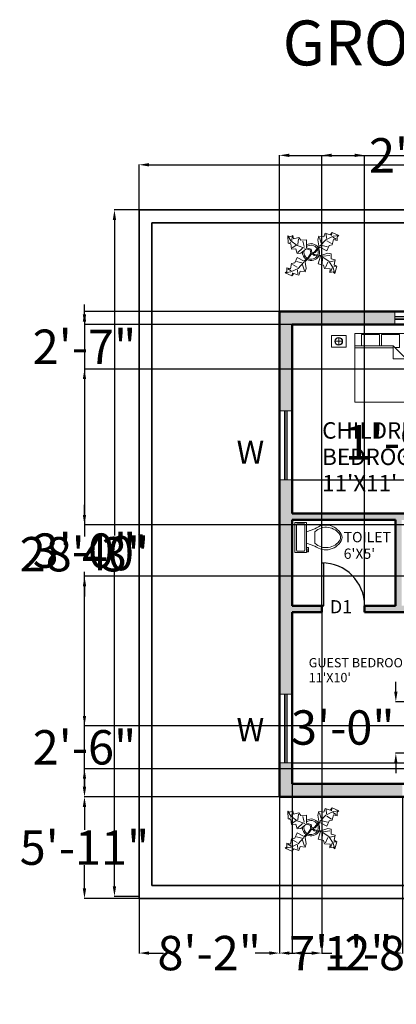
# Model space of a CAD drawing. Units: inches. Extents: x -166 to 1001, y 0 to 688.
# Tile 1 of 11: x -166 to 97, y 0 to 688. Entities that reach past the tile are written whole.
import ezdxf

# ---------------------------------------------------------------- set-up
doc = ezdxf.new("R2010")
doc.units = ezdxf.units.IN
doc.header["$MEASUREMENT"] = 0
for name, color, linetype, lineweight in [('A-ANNO-DIMS', 1, 'Continuous', 18), ('A-ANNO-TEXT', 2, 'Continuous', 25), ('A-AREA-IDEN', 2, 'Continuous', 25), ('A-DOOR', 6, 'Continuous', 25), ('A-FLOR-FIXT', 11, 'Continuous', 18), ('A-GLAZ', 130, 'Continuous', 18), ('A-WALL-PATT', 5, 'Continuous', 13), ('C-SITE-WALL', 250, 'Continuous', 35), ('FURNITURE', 11, 'Continuous', 18), ('TREES', 80, 'Continuous', 13), ('WALLS', 250, 'Continuous', 50)]:
    doc.layers.add(name, color=color, linetype=linetype, lineweight=lineweight)
doc.styles.get("Standard").update_dxf_attribs({"font": 'arial.ttf'})
doc.dimstyles.get("Standard").update_dxf_attribs({"dimtxt": 24, "dimasz": 7, "dimexe": 0.18, "dimexo": 0.0625, "dimgap": 0.09, "dimtad": 0, "dimtih": 1, "dimtoh": 1, "dimdec": 0, "dimzin": 0, "dimdsep": 46, "dimlunit": 3, "dimtxsty": 'Standard', "dimcen": 0.09, "dimadec": 0, "dimazin": 0, "dimtfac": 1, "dimtdec": 0, "dimtofl": 0, "dimtmove": 0, "dimatfit": 3, "dimfxl": 1, "dimtolj": 1, "dimtzin": 0, "dimarcsym": 0})

# ---------------------------------------------------------------- blocks, each defined once
blk = doc.blocks.new('*U6')
for p, q in [((0, 0), (0, -6)), ((40, 0), (40, -6))]:
    blk.add_line(p, q)
blk.add_lwpolyline([(0, 0), (0, 40), (1.75, 40), (1.75, 0)], close=True)
blk.add_arc((0, 0), 40, 0, 90)
blk = doc.blocks.new('Bed - Queen')
for p, q in [((0, -80.00003), (0, 0)), ((0, 0), (59.99999, 0)), ((59.99999, 0), (59.99999, -80.00003)), ((7.99999, -1.2), (28.79998, -1.2)), ((7.99999, -14.4), (7.99999, -1.2)), ((28.79998, -1.2), (28.79998, -14.4)), ((31.19999, -1.2), (51.99999, -1.2)), ((31.19999, -14.4), (31.19999, -1.2)), ((51.99999, -1.2), (51.99999, -16.4)), ((0, -14.4), (44.8, -14.4)), ((44.8, -16.8), (0, -16.8)), ((59.99999, -29.6), (44.8, -14.4)), ((44.8, -14.4), (44.8, -29.6)), ((51.99999, -16.4), (46.79936, -16.4)), ((44.8, -29.6), (59.99999, -29.6)), ((59.99999, -80.00003), (0, -80.00003))]:
    blk.add_line(p, q)
blk = doc.blocks.new('Toilet - top')
for p, q in [((9.5, -6), (9.5, -2)), ((-10, -8.5), (-8, -8.5)), ((-10, -9.5), (-10, -8.5)), ((-7, -9.5), (-10, -9.5)), ((-8, -8.5), (-8, -8)), ((-7, -8), (-7, -9.5)), ((-4, -8), (-6, -14)), ((4, -8), (6, -14)), ((4, -14), (-4, -14))]:
    blk.add_line(p, q)
blk.add_lwpolyline([(10.5, -8), (10.5, 0), (-10.5, 0), (-10.5, -8)], close=True)
for points in [[(-9.5, -2), (-9.5, -6)], [(8.5, -1), (-8.5, -1)], [(-8.5, -7), (8.5, -7)]]:
    blk.add_lwpolyline(points)
for centre, radius, start, end in [((-8.62, -1.88), 0.884, 81.8699, 188.1301), ((-8.62, -6.12), 0.884, 171.8699, 278.1301), ((8.62, -1.88), 0.884, 351.8699, 98.1301), ((8.62, -6.12), 0.884, 261.8699, 8.1301), ((3.52, -21.58), 12.17, 141.46911, 247.97143), ((4.2, -21.82), 11.33, 136.36773, 238.94682), ((-3.52, -21.58), 12.17, 292.02843, 38.53071), ((-4.2, -21.82), 11.33, 301.05301, 43.63209), ((0, -27.88), 4, 245.73182, 294.26817), ((0, -29), 4, 254.86053, 285.13947)]:
    blk.add_arc(centre, radius, start, end)
blk = doc.blocks.new('Plant - Rubber or Philodendron')
for p, q in [((13.3837, 12.301), (14.68, 13.9039)), ((14.68, 13.9039), (19.3848, 11.8146)), ((-16.2005, 11.4774), (-13.9899, 8.1064)), ((-16.2005, 11.4774), (-14.8639, 10.7964)), ((-16.0159, 6.3329), (-16.2005, 11.4774)), ((-15.3434, 6.5514), (-13.9984, 6.9884)), ((-14.8639, 10.7964), (-12.6195, 11.8975)), ((-13.9899, 8.1064), (-9.5434, 4.7185)), ((-13.3174, 8.325), (-13.0735, 11.0065)), ((-12.6195, 11.8975), (-12.1909, 9.4345)), ((-12.1909, 9.4345), (-8.3829, 10.3)), ((-8.8369, 9.409), (-9.0894, 5.6095)), ((-8.3829, 10.3), (-7.0549, 8.501)), ((-7.0549, 8.501), (-3.0284, 8.6941)), ((-4.8529, 4.012), (-5.7184, 7.82)), ((-3.0284, 8.6941), (-3.0709, 3.1041)), ((4.6914, 8.8812), (5.3859, 11.2828)), ((4.6914, 8.8812), (5.5014, 4.4831)), ((5.3859, 11.2828), (8.8871, 10.7908)), ((5.9878, 10.4842), (7.1971, 6.3869)), ((10.3916, 8.7942), (6.2847, 4.4028)), ((8.8871, 10.7908), (9.9809, 13.4933)), ((9.9809, 13.4933), (13.3837, 12.301)), ((15.3859, 11.3055), (10.3916, 8.7942)), ((10.5828, 12.6946), (10.8893, 9.7953)), ((14.2977, 6.1031), (10.9934, 7.9956)), ((14.5816, 13.2037), (14.3848, 11.8033)), ((15.7909, 9.1065), (14.8995, 5.3044)), ((15.2875, 10.6053), (17.5907, 9.2105)), ((19.3848, 11.8146), (15.3859, 11.3055)), ((18.1925, 8.4119), (15.7909, 9.1065)), ((19.3848, 11.8146), (18.1868, 10.9119)), ((18.1868, 10.9119), (18.1925, 8.4119)), ((-14.0069, 5.8704), (-16.0159, 6.3329)), ((-13.5868, 2.2894), (-14.0069, 5.8704)), ((-10.6784, 2.491), (-13.5868, 2.2894)), ((-13.1329, 3.1804), (-10.6614, 4.727)), ((-9.5858, -0.8715), (-10.6784, 2.491)), ((-9.5434, 4.7185), (-4.1917, 2.9888)), ((-9.1318, 0.0195), (-5.9793, 2.9025)), ((-7.1228, -0.443), (-3.5248, 2.2131)), ((-3.5248, 2.2131), (-3.3011, 2.4355)), ((-3.3011, 2.4355), (-0.5306, 1.7947)), ((-3.0709, 3.1041), (0.0797, 2.3163)), ((-0.5306, 1.7947), (-0.2255, -0.5527)), ((-0.5306, 1.7947), (-0.5306, 1.7947)), ((0.0797, 2.3163), (0.4866, -0.031)), ((0.4866, -0.031), (2.1141, 0.2298)), ((2.1141, 0.2298), (5.4346, 3.9146)), ((6.1032, 3.6844), (2.8262, -0.031)), ((5.4346, 3.9146), (5.5014, 4.4831)), ((11.1089, 1.1958), (6.1032, 3.6844)), ((7.7005, 4.8881), (11.5025, 3.9967)), ((12.7005, 4.8994), (11.1089, 1.1958)), ((14.8995, 5.3044), (12.7005, 4.8994)), ((-11.3237, -7.2629), (-9.7321, -3.5593)), ((-6.3237, -7.2516), (-10.1257, -6.3602)), ((-9.7321, -3.5593), (-4.7264, -6.0479)), ((-7.1228, -0.443), (-9.5858, -0.8715)), ((-9.0148, -11.1577), (-4.9047, -6.8122)), ((-2.019, -3.6148), (-4.7264, -6.0479)), ((-4.1246, -6.8466), (-4.0579, -6.2781)), ((-3.3146, -11.2447), (-4.1246, -6.8466)), ((-4.0579, -6.2781), (-0.9375, -3.1608)), ((-2.019, -3.6148), (-0.2255, -0.5527)), ((-0.9375, -3.1608), (0.5883, -0.8135)), ((0.5883, -0.8135), (2.2447, -2.0916)), ((2.8262, -0.031), (1.3003, -0.5527)), ((1.3003, -0.5527), (2.4193, -1.4655)), ((2.2447, -2.0916), (6.7108, -2.6626)), ((2.4193, -1.4655), (6.895, -2.1175)), ((4.943, -7.9659), (6.7108, -2.6626)), ((11.6605, -0.5413), (6.895, -2.1175)), ((12.3677, -6.1981), (7.219, -2.6772)), ((8.125, -4.0768), (7.7715, -7.9659)), ((8.3544, -2.7453), (13.1973, -2.1704)), ((11.6605, -0.5413), (14.1354, -0.8948)), ((15.5496, -10.7943), (12.3677, -6.1981)), ((16.2567, -5.8446), (13.4283, -6.5517)), ((14.1354, -0.8948), (14.1354, -4.4304)), ((14.1354, -4.4304), (16.9638, -5.1375)), ((16.9638, -5.1375), (16.2567, -8.673)), ((-18.008, -14.1781), (-16.8101, -13.2754)), ((-18.008, -14.1781), (-14.0091, -13.669)), ((-16.8157, -10.7754), (-14.4141, -11.4699)), ((-16.8101, -13.2754), (-16.8157, -10.7754)), ((-13.9107, -12.9688), (-16.2139, -11.574)), ((-14.4141, -11.4699), (-13.5228, -7.6679)), ((-14.0091, -13.669), (-9.0148, -11.1577)), ((-13.5228, -7.6679), (-11.3237, -7.2629)), ((-12.921, -8.4665), (-9.6166, -10.359)), ((-9.206, -15.0581), (-9.5126, -12.1588)), ((-7.5103, -13.1543), (-8.6042, -15.8568)), ((-4.0092, -13.6463), (-7.5103, -13.1543)), ((-4.611, -12.8477), (-5.8203, -8.7504)), ((-3.3146, -11.2447), (-4.0092, -13.6463)), ((8.8321, -9.0266), (4.943, -7.9659)), ((9.5392, -11.1479), (8.8321, -9.0266)), ((13.4283, -11.5015), (9.5392, -11.1479)), ((10.2463, -10.4408), (11.6605, -6.9053)), ((13.0748, -13.9763), (13.4283, -11.5015)), ((15.5496, -13.6228), (13.0748, -13.9763)), ((14.8425, -10.7943), (13.7819, -13.2692)), ((16.6103, -14.6834), (15.5496, -10.7943)), ((16.6103, -14.6834), (15.5496, -13.6228)), ((17.3174, -9.7337), (15.9032, -9.7337)), ((16.2567, -8.673), (18.0245, -9.7337)), ((18.0245, -9.7337), (16.6103, -14.6834)), ((-13.3032, -16.2674), (-18.008, -14.1781)), ((-12.0069, -14.6645), (-13.3032, -16.2674)), ((-13.2048, -15.5672), (-13.008, -14.1668)), ((-8.6042, -15.8568), (-12.0069, -14.6645))]:
    blk.add_line(p, q)
for centre, radius, start, end in [((0.0308, 0.1664), 6, 178.6147, 235.1169), ((0.0308, 0.1664), 5, 168.1647, 238.6725), ((0, 0), 6.1275, 34.37569, 120.1028), ((-0.0601, -0.2075), 5.2461, 33.82192, 124.9414), ((-0.2664, 0.1682), 5.2775, 338.4094, 20.03007), ((-0.098, 0.1364), 6.1288, 341.2017, 26.09184), ((-0.0234, 0.3825), 6.1492, 242.5812, 331.2714), ((-0.1102, 0.4886), 5.2883, 247.3711, 327.472)]:
    blk.add_arc(centre, radius, start, end)
blk = doc.blocks.new('*D10')
at = {"layer": 'A-ANNO-DIMS', "color": 0, "lineweight": -2, "transparency": 16777216}
for p, q in [((-82.62, 554.8), (-82.62, 586.48)), ((-75.62, 586.3), (256.61, 586.3)), ((629.88, 586.3), (297.65, 586.3)), ((636.88, 554.8), (636.88, 586.48))]:
    blk.add_line(p, q, dxfattribs=at)
at = {"layer": 'A-ANNO-DIMS', "color": 0, "transparency": 16777216}
for points in [[(-75.62, 587.47), (-75.62, 585.14), (-82.62, 586.3)], [(629.88, 587.47), (629.88, 585.14), (636.88, 586.3)]]:
    blk.add_solid(points, dxfattribs=at)
at = {"layer": 'Defpoints', "color": 0, "transparency": 16777216}
for p in [(636.88, 586.3), (-82.62, 554.74), (636.88, 554.74)]:
    blk.add_point(p, dxfattribs=at)
at = {"layer": 'A-ANNO-DIMS', "color": 0, "transparency": 16777216, "insert": (277.13, 586.3), "char_height": 24, "attachment_point": 5}
blk.add_mtext("\\A1;60'", dxfattribs=at)
blk = doc.blocks.new('*D11')
at = {"layer": 'A-ANNO-DIMS', "color": 0, "lineweight": -2, "transparency": 16777216}
for p, q in [((-82.68, 554.74), (-100.02, 554.74)), ((-99.84, 547.74), (-99.84, 327.33)), ((-99.84, 82.23), (-99.84, 302.64)), ((-82.68, 75.23), (-100.02, 75.23))]:
    blk.add_line(p, q, dxfattribs=at)
at = {"layer": 'A-ANNO-DIMS', "color": 0, "transparency": 16777216}
for points in [[(-101.01, 547.74), (-98.67, 547.74), (-99.84, 554.74)], [(-101.01, 82.23), (-98.67, 82.23), (-99.84, 75.23)]]:
    blk.add_solid(points, dxfattribs=at)
at = {"layer": 'Defpoints', "color": 0, "transparency": 16777216}
for p in [(-82.62, 554.74), (-99.84, 75.23), (-82.62, 75.23)]:
    blk.add_point(p, dxfattribs=at)
at = {"layer": 'A-ANNO-DIMS', "color": 0, "transparency": 16777216, "insert": (-99.84, 314.99), "char_height": 24, "attachment_point": 5}
blk.add_mtext("\\A1;40'", dxfattribs=at)
blk = doc.blocks.new('WIN-48IN')
for p, q in [((0, 4.5), (0, 9)), ((0, 9), (0, 0)), ((48, 9), (48, 0)), ((0, 5.5), (48, 5.5)), ((0, 4.5), (48, 4.5)), ((0, 3.5), (48, 3.5))]:
    blk.add_line(p, q)
blk = doc.blocks.new('BEDSIDE-TABLE-LAMP')
for p, q in [((2.75, 4.1), (7.66, 4.1)), ((5.2, 1.64), (5.2, 6.55))]:
    blk.add_line(p, q)
blk.add_lwpolyline([(0, 8.19), (10.4, 8.19), (10.4, 0), (0, 0)], close=True)
for radius in [2.71, 2.71, 2.71, 2.46]:
    blk.add_circle((5.2, 4.1), radius)
blk = doc.blocks.new('*D24')
at = {"layer": 'A-ANNO-DIMS', "color": 0, "lineweight": -2, "transparency": 16777216}
for p, q in [((96.72, 218.18), (96.72, 225.18)), ((103.86, 211.18), (96.54, 211.18)), ((103.86, 175.18), (96.54, 175.18)), ((96.72, 168.18), (96.72, 161.18))]:
    blk.add_line(p, q, dxfattribs=at)
at = {"layer": 'A-ANNO-DIMS', "color": 0, "transparency": 16777216}
for points in [[(95.56, 218.18), (97.89, 218.18), (96.72, 211.18)], [(95.56, 168.18), (97.89, 168.18), (96.72, 175.18)]]:
    blk.add_solid(points, dxfattribs=at)
at = {"layer": 'Defpoints', "color": 0, "transparency": 16777216}
for p in [(103.92, 211.18), (96.72, 175.18), (103.92, 175.18)]:
    blk.add_point(p, dxfattribs=at)
at = {"layer": 'A-ANNO-DIMS', "color": 0, "transparency": 16777216, "insert": (96.72, 193.18), "char_height": 24, "attachment_point": 5}
blk.add_mtext('\\A1;3\'-0" TYP.', dxfattribs=at)
blk = doc.blocks.new('*D26')
at = {"layer": 'A-ANNO-DIMS', "color": 0, "lineweight": -2, "transparency": 16777216}
for p, q in [((218.29, 420.4), (213.22, 420.4)), ((213.4, 413.4), (213.4, 406.4)), ((218.29, 399.4), (213.22, 399.4)), ((213.4, 399.4), (213.4, 392.4)), ((213.4, 392.4), (206.4, 392.4))]:
    blk.add_line(p, q, dxfattribs=at)
at = {"layer": 'A-ANNO-DIMS', "color": 0, "transparency": 16777216}
for points in [[(212.23, 413.4), (214.57, 413.4), (213.4, 420.4)], [(212.23, 406.4), (214.57, 406.4), (213.4, 399.4)]]:
    blk.add_solid(points, dxfattribs=at)
at = {"layer": 'Defpoints', "color": 0, "transparency": 16777216}
for p in [(218.36, 420.4), (213.4, 399.4), (218.36, 399.4)]:
    blk.add_point(p, dxfattribs=at)
at = {"layer": 'A-ANNO-DIMS', "color": 0, "transparency": 16777216, "insert": (134.29, 392.4), "char_height": 24, "attachment_point": 5}
blk.add_mtext('\\A1;1\'-9" TYP.', dxfattribs=at)
blk = doc.blocks.new('*D35')
at = {"layer": 'A-ANNO-DIMS', "color": 0, "lineweight": -2, "transparency": 16777216}
for p, q in [((15.38, 483.8), (15.38, 593.07)), ((22.38, 592.89), (207.38, 592.89)), ((531.88, 592.89), (346.89, 592.89)), ((538.88, 483.8), (538.88, 593.07))]:
    blk.add_line(p, q, dxfattribs=at)
at = {"layer": 'A-ANNO-DIMS', "color": 0, "transparency": 16777216}
for points in [[(22.38, 594.06), (22.38, 591.72), (15.38, 592.89)], [(531.88, 594.06), (531.88, 591.72), (538.88, 592.89)]]:
    blk.add_solid(points, dxfattribs=at)
at = {"layer": 'Defpoints', "color": 0, "transparency": 16777216}
for p in [(538.88, 592.89), (15.38, 483.74), (538.88, 483.74)]:
    blk.add_point(p, dxfattribs=at)
at = {"layer": 'A-ANNO-DIMS', "color": 0, "transparency": 16777216, "insert": (277.13, 592.89), "char_height": 24, "attachment_point": 5}
blk.add_mtext('\\A1;43\'-7 1/2"', dxfattribs=at)
blk = doc.blocks.new('*D36')
at = {"layer": 'A-ANNO-DIMS', "color": 0, "lineweight": -2, "transparency": 16777216}
for p, q in [((15.32, 483.74), (-120.95, 483.74)), ((-120.77, 476.74), (-120.77, 326.59)), ((-120.77, 151.74), (-120.77, 301.89)), ((15.32, 144.74), (-120.95, 144.74))]:
    blk.add_line(p, q, dxfattribs=at)
at = {"layer": 'A-ANNO-DIMS', "color": 0, "transparency": 16777216}
for points in [[(-121.93, 476.74), (-119.6, 476.74), (-120.77, 483.74)], [(-121.93, 151.74), (-119.6, 151.74), (-120.77, 144.74)]]:
    blk.add_solid(points, dxfattribs=at)
at = {"layer": 'Defpoints', "color": 0, "transparency": 16777216}
for p in [(-120.77, 483.74), (15.38, 483.74), (15.38, 144.74)]:
    blk.add_point(p, dxfattribs=at)
at = {"layer": 'A-ANNO-DIMS', "color": 0, "transparency": 16777216, "insert": (-120.77, 314.24), "char_height": 24, "attachment_point": 5}
blk.add_mtext('\\A1;28\'-3"', dxfattribs=at)
blk = doc.blocks.new('*D37')
at = {"layer": 'A-ANNO-DIMS', "color": 0, "lineweight": -2, "transparency": 16777216}
for p, q in [((15.38, 144.68), (15.38, 35.41)), ((-82.62, 73.68), (-82.62, 35.41)), ((-75.62, 35.59), (-65.62, 35.59)), ((8.38, 35.59), (-1.61, 35.59))]:
    blk.add_line(p, q, dxfattribs=at)
at = {"layer": 'A-ANNO-DIMS', "color": 0, "transparency": 16777216}
for points in [[(-75.62, 36.76), (-75.62, 34.42), (-82.62, 35.59)], [(8.38, 36.76), (8.38, 34.42), (15.38, 35.59)]]:
    blk.add_solid(points, dxfattribs=at)
at = {"layer": 'Defpoints', "color": 0, "transparency": 16777216}
for p in [(15.38, 144.74), (-82.62, 73.74), (15.38, 35.59)]:
    blk.add_point(p, dxfattribs=at)
at = {"layer": 'A-ANNO-DIMS', "color": 0, "transparency": 16777216, "insert": (-33.62, 35.59), "char_height": 24, "attachment_point": 5}
blk.add_mtext('\\A1;8\'-2"', dxfattribs=at)
blk = doc.blocks.new('*D38')
at = {"layer": 'A-ANNO-DIMS', "color": 0, "lineweight": -2, "transparency": 16777216}
for p, q in [((15.32, 144.74), (-120.95, 144.74)), ((-120.77, 137.74), (-120.77, 121.58)), ((-120.77, 80.74), (-120.77, 96.9)), ((-82.68, 73.74), (-120.95, 73.74))]:
    blk.add_line(p, q, dxfattribs=at)
at = {"layer": 'A-ANNO-DIMS', "color": 0, "transparency": 16777216}
for points in [[(-121.93, 137.74), (-119.6, 137.74), (-120.77, 144.74)], [(-121.93, 80.74), (-119.6, 80.74), (-120.77, 73.74)]]:
    blk.add_solid(points, dxfattribs=at)
at = {"layer": 'Defpoints', "color": 0, "transparency": 16777216}
for p in [(-120.77, 144.74), (15.38, 144.74), (-82.62, 73.74)]:
    blk.add_point(p, dxfattribs=at)
at = {"layer": 'A-ANNO-DIMS', "color": 0, "transparency": 16777216, "insert": (-120.77, 109.24), "char_height": 24, "attachment_point": 5}
blk.add_mtext('\\A1;5\'-11"', dxfattribs=at)
blk = doc.blocks.new('*D48')
at = {"layer": 'A-ANNO-DIMS', "color": 0, "lineweight": -2, "transparency": 16777216}
for p, q in [((15.38, 144.68), (15.38, 35.41)), ((101.31, 144.68), (101.31, 35.41)), ((22.38, 35.59), (26.46, 35.59)), ((94.31, 35.59), (90.24, 35.59))]:
    blk.add_line(p, q, dxfattribs=at)
at = {"layer": 'A-ANNO-DIMS', "color": 0, "transparency": 16777216}
for points in [[(22.38, 36.76), (22.38, 34.42), (15.38, 35.59)], [(94.31, 36.76), (94.31, 34.42), (101.31, 35.59)]]:
    blk.add_solid(points, dxfattribs=at)
at = {"layer": 'Defpoints', "color": 0, "transparency": 16777216}
for p in [(15.38, 144.74), (101.31, 144.74), (101.31, 35.59)]:
    blk.add_point(p, dxfattribs=at)
at = {"layer": 'A-ANNO-DIMS', "color": 0, "transparency": 16777216, "insert": (58.35, 35.59), "char_height": 24, "attachment_point": 5}
blk.add_mtext('\\A1;7\'-2"', dxfattribs=at)
blk = doc.blocks.new('*D51')
at = {"layer": 'A-ANNO-DIMS', "color": 0, "lineweight": -2, "transparency": 16777216}
for p, q in [((675.03, 168.41), (675.03, 175.41)), ((675.03, 175.41), (682.03, 175.41)), ((24.44, 168.41), (675.21, 168.41)), ((675.03, 160.74), (675.03, 161.41)), ((24.44, 153.74), (675.21, 153.74))]:
    blk.add_line(p, q, dxfattribs=at)
at = {"layer": 'A-ANNO-DIMS', "color": 0, "transparency": 16777216}
for points in [[(673.87, 161.41), (676.2, 161.41), (675.03, 168.41)], [(673.87, 160.74), (676.2, 160.74), (675.03, 153.74)]]:
    blk.add_solid(points, dxfattribs=at)
at = {"layer": 'Defpoints', "color": 0, "transparency": 16777216}
for p in [(24.38, 168.41), (675.03, 168.41), (24.38, 153.74)]:
    blk.add_point(p, dxfattribs=at)
at = {"layer": 'A-ANNO-DIMS', "color": 0, "transparency": 16777216, "insert": (740.85, 175.41), "char_height": 24, "attachment_point": 5}
blk.add_mtext('\\A1;1\'-2 1/2"', dxfattribs=at)
blk = doc.blocks.new('*D52')
at = {"layer": 'A-ANNO-DIMS', "color": 0, "lineweight": -2, "transparency": 16777216}
for p, q in [((675.03, 366.29), (675.03, 373.29)), ((675.03, 373.29), (682.03, 373.29)), ((24.44, 366.29), (675.21, 366.29)), ((675.03, 349.74), (675.03, 359.29)), ((24.44, 342.74), (675.21, 342.74))]:
    blk.add_line(p, q, dxfattribs=at)
at = {"layer": 'A-ANNO-DIMS', "color": 0, "transparency": 16777216}
for points in [[(673.87, 359.29), (676.2, 359.29), (675.03, 366.29)], [(673.87, 349.74), (676.2, 349.74), (675.03, 342.74)]]:
    blk.add_solid(points, dxfattribs=at)
at = {"layer": 'Defpoints', "color": 0, "transparency": 16777216}
for p in [(24.38, 366.29), (675.03, 366.29), (24.38, 342.74)]:
    blk.add_point(p, dxfattribs=at)
at = {"layer": 'A-ANNO-DIMS', "color": 0, "transparency": 16777216, "insert": (750.18, 373.29), "char_height": 24, "attachment_point": 5}
blk.add_mtext('\\A1;1\'-11 1/2"', dxfattribs=at)
blk = doc.blocks.new('*D55')
at = {"layer": 'A-ANNO-DIMS', "color": 0, "lineweight": -2, "transparency": 16777216}
for p, q in [((-120.77, 341.73), (-120.77, 348.73)), ((529.82, 334.73), (-120.95, 334.73)), ((529.82, 298.79), (-120.95, 298.79)), ((-120.77, 291.79), (-120.77, 284.79))]:
    blk.add_line(p, q, dxfattribs=at)
at = {"layer": 'A-ANNO-DIMS', "color": 0, "transparency": 16777216}
for points in [[(-121.93, 341.73), (-119.6, 341.73), (-120.77, 334.73)], [(-121.93, 291.79), (-119.6, 291.79), (-120.77, 298.79)]]:
    blk.add_solid(points, dxfattribs=at)
at = {"layer": 'Defpoints', "color": 0, "transparency": 16777216}
for p in [(-120.77, 334.73), (529.88, 334.73), (529.88, 298.79)]:
    blk.add_point(p, dxfattribs=at)
at = {"layer": 'A-ANNO-DIMS', "color": 0, "transparency": 16777216, "insert": (-120.77, 316.76), "char_height": 24, "attachment_point": 5}
blk.add_mtext('\\A1;3\'-0"', dxfattribs=at)
blk = doc.blocks.new('*D67')
at = {"layer": 'A-ANNO-DIMS', "color": 0, "lineweight": -2, "transparency": 16777216}
for p, q in [((44.93, 278.3), (44.93, 593.07)), ((51.93, 592.89), (67.93, 592.89)), ((74.93, 278.3), (74.93, 593.07)), ((74.93, 592.89), (81.93, 592.89))]:
    blk.add_line(p, q, dxfattribs=at)
at = {"layer": 'A-ANNO-DIMS', "color": 0, "transparency": 16777216}
for points in [[(51.93, 594.06), (51.93, 591.72), (44.93, 592.89)], [(67.93, 594.06), (67.93, 591.72), (74.93, 592.89)]]:
    blk.add_solid(points, dxfattribs=at)
at = {"layer": 'Defpoints', "color": 0, "transparency": 16777216}
for p in [(74.93, 592.89), (44.93, 278.24), (74.93, 278.24)]:
    blk.add_point(p, dxfattribs=at)
at = {"layer": 'A-ANNO-DIMS', "color": 0, "transparency": 16777216, "insert": (114.12, 592.89), "char_height": 24, "attachment_point": 5}
blk.add_mtext('\\A1;2\'-6"', dxfattribs=at)
blk = doc.blocks.new('*D68')
at = {"layer": 'A-ANNO-DIMS', "color": 0, "lineweight": -2, "transparency": 16777216}
for p, q in [((24.38, 273.68), (24.38, 35.41)), ((44.93, 273.68), (44.93, 35.41)), ((31.38, 35.59), (37.93, 35.59)), ((44.93, 35.59), (51.93, 35.59))]:
    blk.add_line(p, q, dxfattribs=at)
at = {"layer": 'A-ANNO-DIMS', "color": 0, "transparency": 16777216}
for points in [[(31.38, 36.76), (31.38, 34.42), (24.38, 35.59)], [(37.93, 36.76), (37.93, 34.42), (44.93, 35.59)]]:
    blk.add_solid(points, dxfattribs=at)
at = {"layer": 'Defpoints', "color": 0, "transparency": 16777216}
for p in [(24.38, 273.74), (44.93, 273.74), (44.93, 35.59)]:
    blk.add_point(p, dxfattribs=at)
at = {"layer": 'A-ANNO-DIMS', "color": 0, "transparency": 16777216, "insert": (110.75, 35.59), "char_height": 24, "attachment_point": 5}
blk.add_mtext('\\A1;1\'-8 1/2"', dxfattribs=at)
blk = doc.blocks.new('*D73')
at = {"layer": 'A-ANNO-DIMS', "color": 0, "lineweight": -2, "transparency": 16777216}
for p, q in [((-120.77, 201.32), (-120.77, 208.32)), ((393.32, 194.32), (-120.95, 194.32)), ((393.32, 164.32), (-120.95, 164.32)), ((-120.77, 157.32), (-120.77, 150.32))]:
    blk.add_line(p, q, dxfattribs=at)
at = {"layer": 'A-ANNO-DIMS', "color": 0, "transparency": 16777216}
for points in [[(-121.93, 201.32), (-119.6, 201.32), (-120.77, 194.32)], [(-121.93, 157.32), (-119.6, 157.32), (-120.77, 164.32)]]:
    blk.add_solid(points, dxfattribs=at)
at = {"layer": 'Defpoints', "color": 0, "transparency": 16777216}
for p in [(-120.77, 194.32), (393.38, 194.32), (393.38, 164.32)]:
    blk.add_point(p, dxfattribs=at)
at = {"layer": 'A-ANNO-DIMS', "color": 0, "transparency": 16777216, "insert": (-120.77, 179.32), "char_height": 24, "attachment_point": 5}
blk.add_mtext('\\A1;2\'-6"', dxfattribs=at)
blk = doc.blocks.new('*D75')
at = {"layer": 'A-ANNO-DIMS', "color": 0, "lineweight": -2, "transparency": 16777216}
for p, q in [((-120.77, 481.74), (-120.77, 488.74)), ((529.82, 474.74), (-120.95, 474.74)), ((529.82, 443.59), (-120.95, 443.59)), ((-120.77, 436.59), (-120.77, 429.59))]:
    blk.add_line(p, q, dxfattribs=at)
at = {"layer": 'A-ANNO-DIMS', "color": 0, "transparency": 16777216}
for points in [[(-121.93, 481.74), (-119.6, 481.74), (-120.77, 474.74)], [(-121.93, 436.59), (-119.6, 436.59), (-120.77, 443.59)]]:
    blk.add_solid(points, dxfattribs=at)
at = {"layer": 'Defpoints', "color": 0, "transparency": 16777216}
for p in [(529.88, 474.74), (-120.77, 443.59), (529.88, 443.59)]:
    blk.add_point(p, dxfattribs=at)
at = {"layer": 'A-ANNO-DIMS', "color": 0, "transparency": 16777216, "insert": (-120.77, 459.16), "char_height": 24, "attachment_point": 5}
blk.add_mtext('\\A1;2\'-7"', dxfattribs=at)

msp = doc.modelspace()

# ---------------------------------------------------------------- hatches: boundary and pattern name
at = {"layer": 'A-WALL-PATT'}
h = msp.add_hatch(color=256, dxfattribs=at)
h.dxf.hatch_style = 1
h.paths.add_polyline_path([(96.05, 483.74), (15.38, 483.74), (15.38, 414.29), (24.38, 414.29), (24.38, 474.74), (96.05, 474.74)])
h.paths.add_polyline_path([(175.47, 483.74), (144.05, 483.74), (144.05, 474.74), (156.38, 474.74), (175.47, 474.74)])
h.paths.add_polyline_path([(298.66, 483.74), (199.47, 483.74), (199.47, 474.74), (256.88, 474.74), (298.66, 474.74)])
h.paths.add_polyline_path([(430.46, 483.74), (346.66, 483.74), (346.66, 474.74), (393.38, 474.74), (430.46, 474.74)])
h.paths.add_polyline_path([(261.38, 474.74), (256.88, 474.74), (256.88, 342.74), (201.55, 342.74), (201.55, 338.24), (274.49, 338.24), (274.49, 342.74), (261.38, 342.74)])
h.paths.add_polyline_path([(160.88, 474.74), (156.38, 474.74), (156.38, 342.74), (146.03, 342.74), (146.03, 338.24), (171.55, 338.24), (171.55, 342.74), (160.88, 342.74)])
h.paths.add_polyline_path([(397.88, 474.74), (393.38, 474.74), (393.38, 383.21), (397.88, 383.21)])
h.paths.add_polyline_path([(538.88, 362.18), (529.88, 362.18), (529.88, 342.74), (397.88, 342.74), (397.88, 348.69), (393.38, 348.69), (393.38, 342.74), (384.24, 342.74), (384.24, 338.24), (529.88, 338.24), (529.88, 334.73), (538.88, 334.73)])
h.paths.add_polyline_path([(538.88, 483.74), (478.46, 483.74), (478.46, 474.74), (529.88, 474.74), (529.88, 410.18), (538.88, 410.18)])
h.paths.add_polyline_path([(538.88, 298.79), (529.88, 298.79), (529.88, 278.24), (442.61, 278.24), (442.61, 273.74), (529.88, 273.74), (529.88, 221.94), (538.88, 221.94)])
h.paths.add_polyline_path([(538.88, 173.94), (529.88, 173.94), (529.88, 153.74), (393.38, 153.74), (382.23, 153.74), (382.23, 144.74), (538.88, 144.74)])
h.paths.add_polyline_path([(397.88, 164.32), (393.38, 164.32), (393.38, 153.74), (397.88, 153.74)], flags=17)
h.paths.add_polyline_path([(397.88, 273.74), (406.66, 273.74), (406.66, 278.24), (393.38, 278.24), (393.38, 273.74), (393.38, 230.24), (316.88, 230.24), (316.88, 153.74), (321.38, 153.74), (321.38, 225.74), (393.38, 225.74), (393.38, 194.32), (397.88, 194.32)])
h.paths.add_polyline_path([(358.23, 153.74), (316.88, 153.74), (284.58, 153.74), (284.58, 144.74), (358.23, 144.74)])
h.paths.add_polyline_path([(224.58, 153.74), (156.38, 153.74), (149.31, 153.74), (149.31, 144.74), (224.58, 144.74)])
h.paths.add_polyline_path([(101.31, 153.74), (24.38, 153.74), (24.38, 168.41), (15.38, 168.41), (15.38, 144.74), (101.31, 144.74)])
h.paths.add_polyline_path([(160.88, 273.74), (160.88, 278.24), (147.87, 278.24), (147.87, 273.74), (156.38, 273.74), (156.38, 153.74), (160.88, 153.74)])
h.paths.add_polyline_path([(111.92, 278.24), (100.88, 278.24), (100.88, 338.24), (110.03, 338.24), (110.03, 342.74), (24.38, 342.74), (24.38, 366.29), (15.38, 366.29), (15.38, 216.41), (24.38, 216.41), (24.38, 273.74), (44.93, 273.74), (44.93, 278.24), (24.38, 278.24), (24.38, 338.24), (96.38, 338.24), (96.38, 278.24), (74.93, 278.24), (74.93, 273.74), (111.92, 273.74)])

# ---------------------------------------------------------------- linework, layer by layer
at = {"layer": 'C-SITE-WALL'}
for p, q in [((-82.62, 554.74), (636.88, 554.74)), ((-82.62, 73.74), (-82.62, 554.74)), ((-73.62, 545.74), (627.88, 545.74)), ((-73.62, 82.74), (-73.62, 545.74)), ((-73.62, 82.74), (627.88, 82.74)), ((-82.62, 73.74), (636.88, 73.74))]:
    msp.add_line(p, q, dxfattribs=at)
at = {"layer": 'WALLS'}
for p, q in [((15.38, 144.74), (15.38, 483.74)), ((15.38, 483.74), (538.88, 483.74)), ((24.38, 474.74), (156.38, 474.74)), ((24.38, 342.74), (24.38, 474.74)), ((24.38, 342.74), (110.03, 342.74)), ((24.38, 338.24), (96.38, 338.24)), ((24.38, 278.24), (24.38, 338.24)), ((96.38, 278.24), (96.38, 338.24)), ((24.38, 278.24), (46.24, 278.24)), ((44.93, 278.24), (44.93, 273.74)), ((74.93, 278.24), (96.38, 278.24)), ((74.93, 273.74), (74.93, 278.24)), ((24.38, 153.74), (24.38, 273.74)), ((24.38, 273.74), (44.93, 273.74)), ((74.93, 273.74), (111.92, 273.74)), ((24.38, 153.74), (156.38, 153.74)), ((15.38, 144.74), (538.88, 144.74))]:
    msp.add_line(p, q, dxfattribs=at)

# ---------------------------------------------------------------- block references
at = {"layer": 'A-DOOR', "xscale": 0.7500000000000006, "yscale": 0.7500000000000006, "zscale": 0.7500000000000006}
msp.add_blockref('*U6', (44.93, 278.24), dxfattribs=at)
at = {"layer": 'A-FLOR-FIXT', "rotation": 90}
msp.add_blockref('Toilet - top', (26.23, 325.94), dxfattribs=at)
at = {"layer": 'A-GLAZ'}
msp.add_blockref('WIN-48IN', (96.05, 474.74), dxfattribs=at)
at = {"layer": 'A-GLAZ', "rotation": 89.99999999999969}
for p in [(24.38, 366.29), (24.38, 168.41)]:
    msp.add_blockref('WIN-48IN', p, dxfattribs=at)
at = {"layer": 'FURNITURE', "xscale": 0.6000001000000168, "yscale": 0.6000001000000168, "zscale": 0.6000001000000168}
msp.add_blockref('Bed - Queen', (68.02, 468.51), dxfattribs=at)
at = {"layer": 'FURNITURE'}
msp.add_blockref('BEDSIDE-TABLE-LAMP', (51.66, 458.89), dxfattribs=at)
at = {"layer": 'TREES'}
for p in [(37.45, 525.09), (37.45, 123.15)]:
    msp.add_blockref('Plant - Rubber or Philodendron', p, dxfattribs=at)

# ---------------------------------------------------------------- texts
at = {"layer": 'A-ANNO-TEXT'}
for s, height, p in [('GROUND FLOOR PLAN', 31.3778, (17.68, 655.72)), ('W ', 16.096, (-14.52, 377.47)), ('D1', 9.17, (50.66, 272.97)), ('W ', 16.096, (-14.52, 183.62))]:
    msp.add_text(s, height=height, dxfattribs=at).set_placement(p)
at = {"layer": 'A-AREA-IDEN'}
for s, height, p in [("CHILDREN'S", 11.478, (45.26, 394.98)), ('BEDROOM', 11.478, (45.26, 376.54)), ("11'X11'", 11.478, (45.26, 358.1)), ('TOILET', 7.198, (60.27, 322.58)), ("6'X5'", 7.198, (60.27, 311.02)), ('GUEST BEDROOM', 6.4554, (35.86, 235.21)), ("11'X10'", 6.455, (35.86, 224.84))]:
    msp.add_text(s, height=height, dxfattribs=at).set_placement(p)

# ---------------------------------------------------------------- dimensions: what is measured, and where the dimension line sits
at = {"layer": 'A-ANNO-DIMS'}
for base, p1, p2, override, picture, middle in [((538.88, 592.89), (15.38, 483.74), (538.88, 483.74), {"dimdec": 1, "dimlfac": 1, "dimrnd": 0, "dimzin": 1, "dimdsep": 46, "dimlunit": 4, "dimfrac": 2}, '*D35', (277.13, 592.89)), ((74.93, 592.89), (44.93, 278.24), (74.93, 278.24), {"dimdec": 1, "dimlfac": 1, "dimrnd": 0, "dimzin": 1, "dimdsep": 46, "dimlunit": 4, "dimfrac": 2}, '*D67', (114.12, 592.89)), ((636.88246038, 586.30455527), (-82.61753962, 554.740867), (636.88246038, 554.740867), {"dimclrd": 0, "dimclre": 0, "dimclrt": 0}, '*D10', (277.13246038, 586.30455527)), ((44.9284, 35.5909), (24.3825, 273.7409), (44.9284, 273.7409), {"dimdec": 1, "dimlfac": 1, "dimrnd": 0, "dimzin": 1, "dimdsep": 46, "dimlunit": 4, "dimfrac": 2}, '*D68', (110.7496, 35.5909)), ((15.38, 35.59), (-82.62, 73.74), (15.38, 144.74), {"dimdec": 1, "dimlfac": 1, "dimrnd": 0, "dimzin": 1, "dimdsep": 46, "dimlunit": 4, "dimfrac": 2}, '*D37', (-33.62, 35.59)), ((101.31, 35.59), (15.38, 144.74), (101.31, 144.74), {"dimdec": 1, "dimlfac": 1, "dimrnd": 0, "dimzin": 1, "dimdsep": 46, "dimlunit": 4, "dimfrac": 2}, '*D48', (58.35, 35.59))]:
    dim = msp.add_linear_dim(base=base, p1=p1, p2=p2, dimstyle='Standard', override=override, dxfattribs=at)
    dim.commit()
    dim.dimension.update_dxf_attribs({"geometry": picture, "text_midpoint": middle})
for base, p1, p2, override, picture, middle in [((-99.84, 75.23), (-82.62, 554.74), (-82.62, 75.23), {"dimclrd": 0, "dimclre": 0, "dimclrt": 0}, '*D11', (-99.84, 314.99)), ((-120.7675, 443.5862), (529.8825, 474.7409), (529.8825, 443.5862), {"dimdec": 1, "dimlfac": 1, "dimrnd": 0, "dimzin": 1, "dimdsep": 46, "dimlunit": 4, "dimfrac": 2}, '*D75', (-120.7675, 459.1635)), ((-120.77, 483.74), (15.38, 144.74), (15.38, 483.74), {"dimdec": 1, "dimlfac": 1, "dimrnd": 0, "dimzin": 1, "dimdsep": 46, "dimlunit": 4, "dimfrac": 2}, '*D36', (-120.77, 314.24)), ((675.0325, 366.2884), (24.3825, 342.7409), (24.3825, 366.2884), {"dimdec": 1, "dimlfac": 1, "dimrnd": 0, "dimzin": 1, "dimdsep": 46, "dimlunit": 4, "dimfrac": 2}, '*D52', (750.177, 373.2884)), ((-120.77, 334.73), (529.88, 298.79), (529.88, 334.73), {"dimdec": 1, "dimlfac": 1, "dimrnd": 0, "dimzin": 1, "dimdsep": 46, "dimlunit": 4, "dimfrac": 2}, '*D55', (-120.77, 316.76)), ((-120.77, 194.32), (393.38, 164.32), (393.38, 194.32), {"dimdec": 1, "dimlfac": 1, "dimrnd": 0, "dimzin": 1, "dimdsep": 46, "dimlunit": 4, "dimfrac": 2}, '*D73', (-120.77, 179.32)), ((675.03, 168.41), (24.38, 153.74), (24.38, 168.41), {"dimdec": 1, "dimlfac": 1, "dimrnd": 0, "dimzin": 1, "dimdsep": 46, "dimlunit": 4, "dimfrac": 2}, '*D51', (740.85, 175.41)), ((-120.77, 144.74), (-82.62, 73.74), (15.38, 144.74), {"dimdec": 1, "dimlfac": 1, "dimrnd": 0, "dimzin": 1, "dimdsep": 46, "dimlunit": 4, "dimfrac": 2}, '*D38', (-120.77, 109.24))]:
    dim = msp.add_linear_dim(base=base, p1=p1, p2=p2, angle=90, dimstyle='Standard', override=override, dxfattribs=at)
    dim.commit()
    dim.dimension.update_dxf_attribs({"geometry": picture, "text_midpoint": middle})
for base, p1, p2, picture, middle in [((213.4, 399.4), (218.36, 420.4), (218.36, 399.4), '*D26', (134.29, 392.4)), ((96.72, 175.18), (103.92, 211.18), (103.92, 175.18), '*D24', (96.72, 193.18))]:
    dim = msp.add_linear_dim(base=base, p1=p1, p2=p2, angle=270, text='<> TYP.', dimstyle='Standard', override={"dimdec": 1, "dimlfac": 1, "dimrnd": 0, "dimzin": 1, "dimdsep": 46, "dimlunit": 4, "dimfrac": 2}, dxfattribs=at)
    dim.commit()
    dim.dimension.update_dxf_attribs({"geometry": picture, "text_midpoint": middle})

doc.saveas('drawing.dxf')
